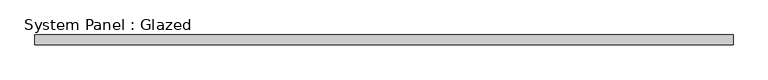
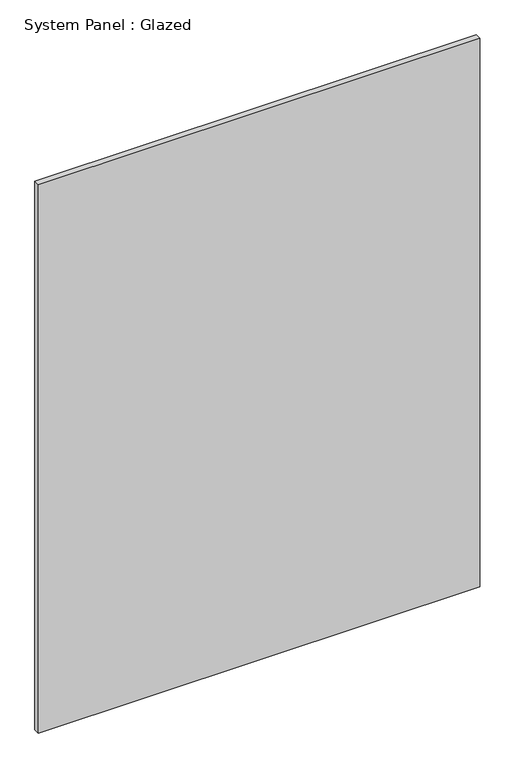
"""IFC4 building model written with IfcOpenShell, lengths in millimetres: plate geometry, System Panel : Glazed."""

from ifc_helpers import new_model, si_unit, origin, origin_with_axes, place, context, project, spatial, polyline, outline, extrude, source, transform, mapped, element, save


def system_panel_glazed_99388aa9(model_context):
    return source(origin(), model_context, "Body", "SweptSolid", [
        extrude(outline(polyline([(890.0, 24.5), (-890.0, 24.5), (-890.0, 49.5), (890.0, 49.5), (890.0, 24.5)])), origin_with_axes(), (0.0, 0.0, 1.0), 2338.4),
    ])


if __name__ == "__main__":
    model = new_model("IFC4")
    model_context = context("Model", 3, world=origin())
    ifc_project = project(units=[si_unit("LENGTHUNIT", "METRE", prefix="MILLI")], contexts=[model_context])
    site = spatial("IfcSite", under=ifc_project)
    building = spatial("IfcBuilding", under=site)
    placement = place(None, origin())
    system_panel_glazed_shape = system_panel_glazed_99388aa9(model_context)
    element("IfcPlate", 1, ObjectType="System Panel : Glazed", at=placement, inside=building, context=model_context, shape_type="MappedRepresentation", body=[
        mapped(system_panel_glazed_shape, transform((0.0, 0.0, 0.0), x_axis=(1.0, 0.0, 0.0), y_axis=(0.0, 1.0, 0.0), z_axis=(0.0, 0.0, 1.0))),
    ])
    save(model, "model.ifc")

# Revit data of these elements
# Type "System Panel : Glazed"
#   Construction Type Id = "GSP4R"
#   Analytic Construction = "1/8 in Pilkington single glazing"
#   Visual Light Transmittance = 0.9
#   Solar Heat Gain Coefficient = 0.86
#   Heat Transfer Coefficient (U) = 6.7069 W/(m²·K)
# Element 1 (IfcPlate, "System Panel : Glazed")
#   Materials on its faces: "Glass"
# Materials
#   "Glass": class "Glass", colour RGB 0 128 192, transparency 0.9, Description = "Soda Lime Glass", Cost = 0
